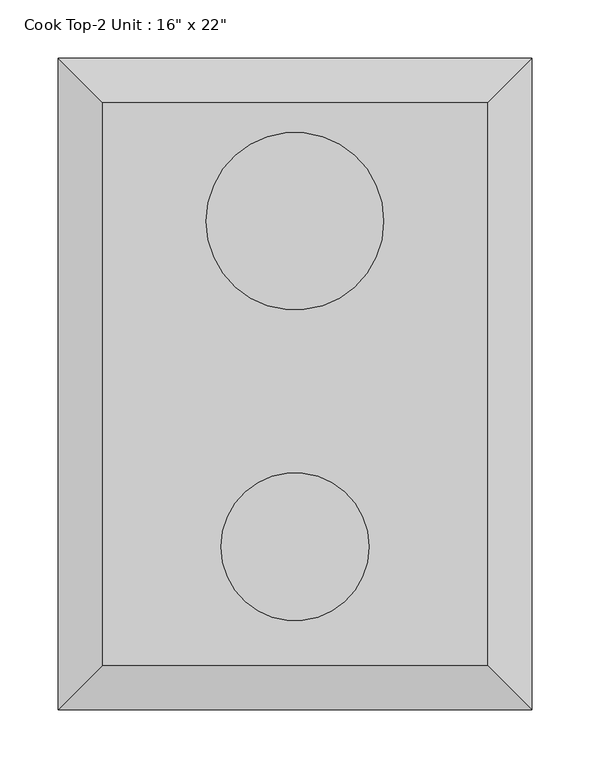
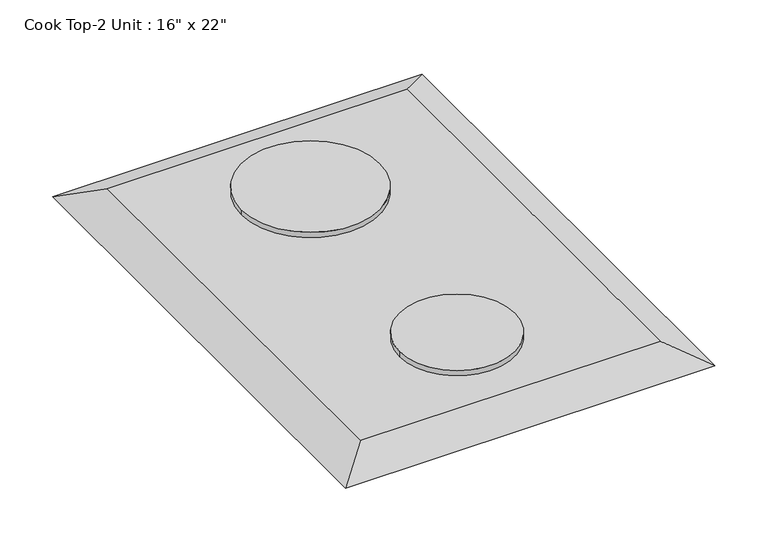
"""IFC4 building model written with IfcOpenShell, lengths in millimetres: proxy geometry."""

from ifc_helpers import new_model, si_unit, point, frame, frame_2d, origin, place, context, project, spatial, circle_curve, trimmed, segment, composite_curve, outline, extrude, faceted_brep, source, transform, mapped, element, save


def proxy_caef4acf(model_context):
    return source(origin(), model_context, "Body", "SolidModel", [
        faceted_brep([(241.3, 271.5247956, 806.45), (-88.9, 271.5247956, 806.45), (-88.9, -211.0752044, 806.45), (241.3, -211.0752044, 806.45), (279.4, 309.6247956, 787.4), (279.4, -249.1752044, 787.4), (-127.0, -249.1752044, 787.4), (-127.0, 309.6247956, 787.4)], [[[0, 1, 2, 3]], [[4, 5, 6, 7]], [[4, 7, 1, 0]], [[7, 6, 2, 1]], [[6, 5, 3, 2]], [[5, 4, 0, 3]]]),
        extrude(outline(composite_curve([segment(trimmed(circle_curve(frame_2d((76.2, 169.9247956)), 76.2), [point((152.4, 169.9247956))], [point((0.0, 169.9247956))], False, "CARTESIAN"), True, "CONTINUOUS"), segment(trimmed(circle_curve(frame_2d((76.2, 169.9247956)), 76.2), [point((0.0, 169.9247956))], [point((152.4, 169.9247956))], False, "CARTESIAN"), True, "CONTINUOUS")], self_intersect=False)), frame((0.0, 0.0, 806.45), z_axis=(0.0, 0.0, 1.0), x_axis=(1.0, 0.0, 0.0)), (0.0, 0.0, 1.0), 6.35),
        extrude(outline(composite_curve([segment(trimmed(circle_curve(frame_2d((76.2, -109.4752044)), 63.5), [point((139.7, -109.4752044))], [point((12.7, -109.4752044))], False, "CARTESIAN"), True, "CONTINUOUS"), segment(trimmed(circle_curve(frame_2d((76.2, -109.4752044)), 63.5), [point((12.7, -109.4752044))], [point((139.7, -109.4752044))], False, "CARTESIAN"), True, "CONTINUOUS")], self_intersect=False)), frame((0.0, 0.0, 806.45), z_axis=(0.0, 0.0, 1.0), x_axis=(1.0, 0.0, 0.0)), (0.0, 0.0, 1.0), 6.35),
    ])


if __name__ == "__main__":
    model = new_model("IFC4")
    model_context = context("Model", 3, world=origin())
    ifc_project = project(units=[si_unit("LENGTHUNIT", "METRE", prefix="MILLI")], contexts=[model_context])
    site = spatial("IfcSite", under=ifc_project)
    building = spatial("IfcBuilding", under=site)
    placement = place(None, origin())
    proxy_shape = proxy_caef4acf(model_context)
    element("IfcBuildingElementProxy", 1, Name="Cook Top-2 Unit : 16\" x 22\"", ObjectType="Cook Top-2 Unit : 16\" x 22\"", at=placement, inside=building, context=model_context, shape_type="MappedRepresentation", body=[
        mapped(proxy_shape, transform((0.0, 0.0, 0.0), x_axis=(1.0, 0.0, 0.0), y_axis=(0.0, 1.0, 0.0), z_axis=(0.0, 0.0, 1.0))),
    ])
    save(model, "model.ifc")

# Revit data of these elements
# Type "Cook Top-2 Unit : 16\" x 22\""
#   Assembly Code = "E1090400"
#   Counter Height = 2' - 7"
#   Depth = 1' - 10"
#   Width = 1' - 4"
#   Burner Material = Metal - Chrome
#   Cooktop Material = Metal - Steel, Polished
#   Default Elevation = 0
# Element 1 (IfcBuildingElementProxy, "Cook Top-2 Unit : 16\" x 22\"")
#   Materials on its faces: "Metal - Steel, Polished", "Metal - Chrome"
# Materials
#   "Metal - Chrome": colour RGB 17 17 17, transparency 0
#   "Metal - Steel, Polished": colour RGB 127 127 127, transparency 0
